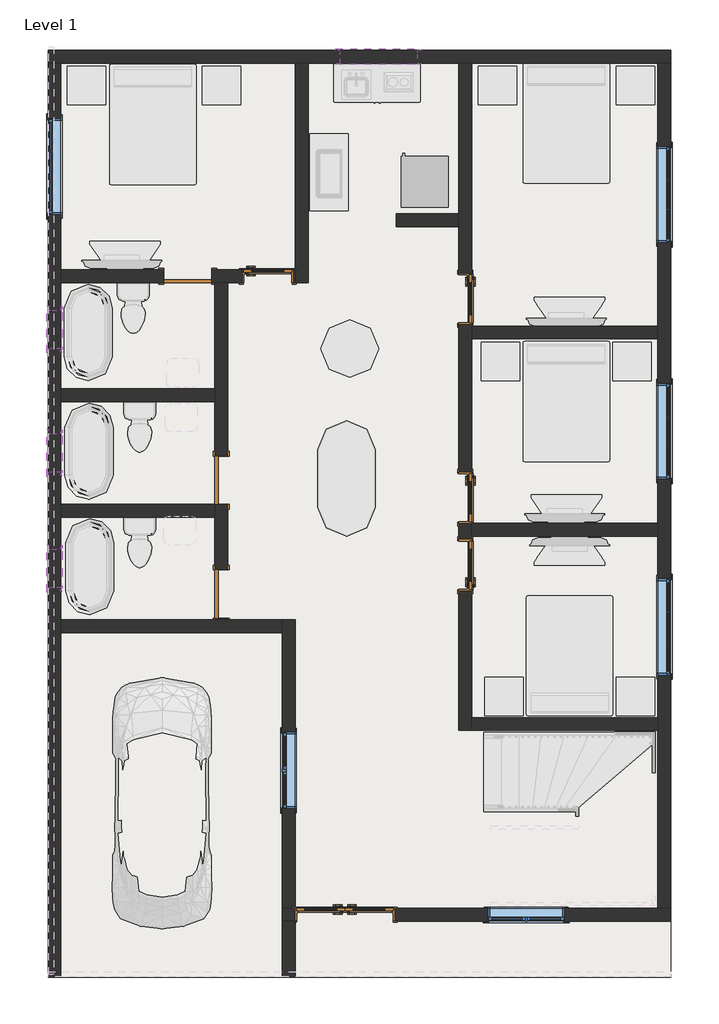
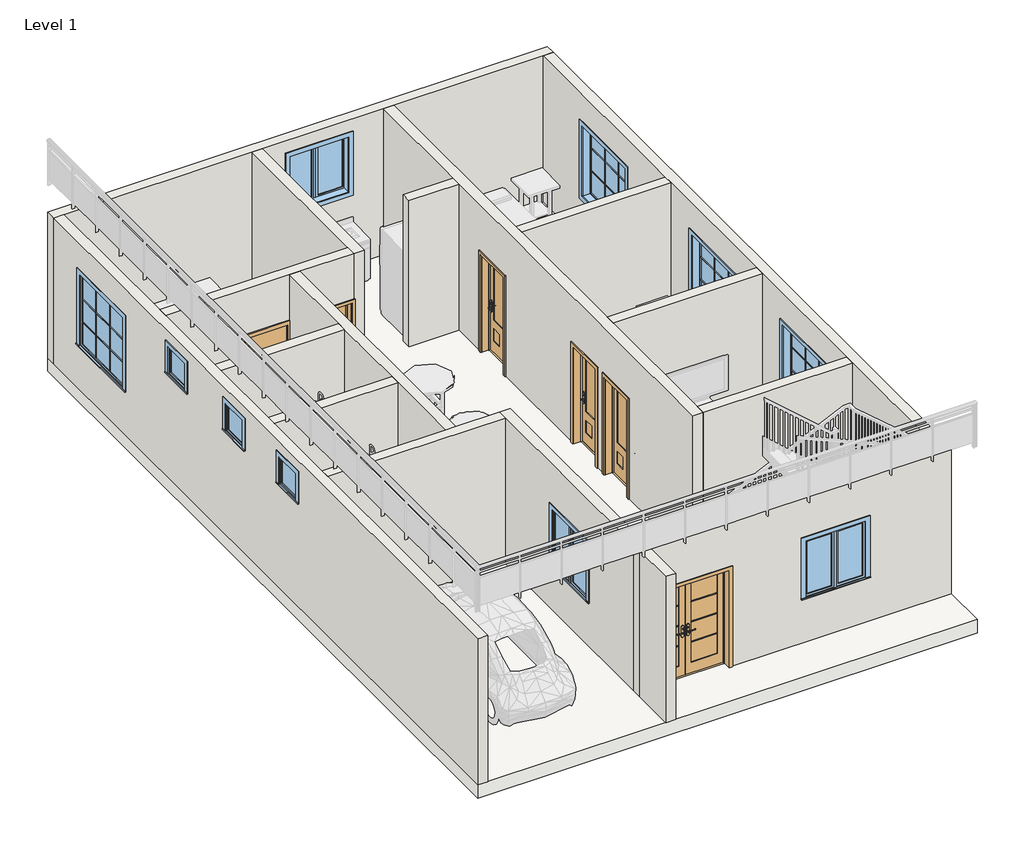
# One storey, part 1 of 4: 17 walls, 10 windows, 8 doors, 1 slab.
"""IFC4 building model written with IfcOpenShell, lengths in millimetres."""

from ifc_helpers import new_model, si_unit, frame, origin, origin_with_axes, place, context, project, spatial, polyline, outline, extrude, faceted_brep, transform, mapped, element, save
from components import door_ad59dcae, door_41326d50, door_b03bd389, door_53b1b562, window_8901c6e2, window_0862ab64, window_e41d21a6

model = new_model("IFC4")

# Units and contexts
model_context = context("Model", 3, world=origin())
ifc_project = project(units=[si_unit("LENGTHUNIT", "METRE", prefix="MILLI")], contexts=[model_context])

# Site, building, storey
site = spatial("IfcSite", under=ifc_project)
building = spatial("IfcBuilding", under=site)
storey = spatial("IfcBuildingStorey", under=building, Name="Level 1", Elevation=0.0)

# Doors
placement = place(None, origin())
door_shape = door_ad59dcae(model_context)
element("IfcDoor", 1, ObjectType="30\" x 80\"", at=placement, inside=storey, context=model_context, shape_type="MappedRepresentation", body=[
    mapped(door_shape, transform((-5611.6297602, 5281.5174997, 0.0), x_axis=(0.0, -1.0, 0.0), y_axis=(1.0, 0.0, 0.0), z_axis=(0.0, 0.0, 1.0))),
])
door_2_shape = door_41326d50(model_context)
element("IfcDoor", 2, ObjectType="30\" x 80\"", at=placement, inside=storey, context=model_context, shape_type="MappedRepresentation", body=[
    mapped(door_2_shape, transform((-5611.6297602, 6348.3174997, 0.0), x_axis=(0.0, 1.0, 0.0), y_axis=(-1.0, 0.0, 0.0), z_axis=(0.0, 0.0, 1.0))),
])
element("IfcDoor", 3, ObjectType="30\" x 80\"", at=placement, inside=storey, context=model_context, shape_type="MappedRepresentation", body=[
    mapped(door_2_shape, transform((-5611.6297602, 9497.9174997, 0.0), x_axis=(0.0, 1.0, 0.0), y_axis=(-1.0, 0.0, 0.0), z_axis=(0.0, 0.0, 1.0))),
])
element("IfcDoor", 4, ObjectType="30\" x 80\"", at=placement, inside=storey, context=model_context, shape_type="MappedRepresentation", body=[
    mapped(door_2_shape, transform((-8739.0047602, 9856.6924997, 0.0), x_axis=(-1.0, 0.0, 0.0), y_axis=(0.0, -1.0, 0.0), z_axis=(0.0, 0.0, 1.0))),
])
door_3_shape = door_b03bd389(model_context)
element("IfcDoor", 5, ObjectType="Door-Exterior-Double-Full Glass-Wood_Clad : 60\" x 80\"", at=placement, inside=storey, context=model_context, shape_type="MappedRepresentation", body=[
    mapped(door_3_shape, transform((-7519.8047602, -252.5075003, 0.0), x_axis=(1.0, 0.0, 0.0), y_axis=(0.0, 1.0, 0.0), z_axis=(0.0, 0.0, 1.0))),
])
door_4_shape = door_53b1b562(model_context)
element("IfcDoor", 6, ObjectType="Single-Flush : 30\" x 80\"", at=placement, inside=storey, context=model_context, shape_type="MappedRepresentation", body=[
    mapped(door_4_shape, transform((-9475.6047602, 4824.3174997, 0.0), x_axis=(0.0, -1.0, 0.0), y_axis=(1.0, 0.0, 0.0), z_axis=(0.0, 0.0, 1.0))),
])
element("IfcDoor", 7, ObjectType="Single-Flush : 30\" x 80\"", at=placement, inside=storey, context=model_context, shape_type="MappedRepresentation", body=[
    mapped(door_4_shape, transform((-9475.6047602, 6627.7174997, 0.0), x_axis=(0.0, -1.0, 0.0), y_axis=(1.0, 0.0, 0.0), z_axis=(0.0, 0.0, 1.0))),
])
element("IfcDoor", 8, ObjectType="Single-Flush : 30\" x 80\"", at=placement, inside=storey, context=model_context, shape_type="MappedRepresentation", body=[
    mapped(door_4_shape, transform((-10009.0047602, 9853.5174997, 0.0), x_axis=(1.0, 0.0, 0.0), y_axis=(0.0, 1.0, 0.0), z_axis=(0.0, 0.0, 1.0))),
])

# Slab
element("IfcSlab", 9, ObjectType="Wood Joist 10\" - Ceramic Tile", at=placement, inside=storey, context=model_context, shape_type="SweptSolid", body=[
    extrude(outline(polyline([(-2363.6047602, 13434.9174997), (-2363.6047602, -357.2825003), (-2363.6047602, -1246.2825003), (-12218.8047602, -1246.2825003), (-12218.8047602, 13434.9174997), (-2363.6047602, 13434.9174997)])), frame((0.0, 0.0, -273.05), z_axis=(0.0, 0.0, 1.0), x_axis=(1.0, 0.0, 0.0)), (0.0, 0.0, 1.0), 273.05),
])

# Walls
element("IfcWall", 10, ObjectType="Generic - 8\"", at=placement, inside=storey, context=model_context, shape_type="Brep", body=[
    faceted_brep([(-12015.6047602, -1246.2825003, 0.0), (-12015.6047602, 4214.7174997, 0.0), (-12015.6047602, 4417.9174997, 0.0), (-12015.6047602, 6043.5174997, 0.0), (-12015.6047602, 6246.7174997, 0.0), (-12015.6047602, 7872.3174997, 0.0), (-12015.6047602, 8075.5174997, 0.0), (-12015.6047602, 9751.9174997, 0.0), (-12015.6047602, 9955.1174997, 0.0), (-12015.6047602, 13231.7174997, 0.0), (-12015.6047602, 13231.7174997, 3048.0), (-12015.6047602, 9955.1174997, 3048.0), (-12015.6047602, 9751.9174997, 3048.0), (-12015.6047602, 8075.5174997, 3048.0), (-12015.6047602, 7872.3174997, 3048.0), (-12015.6047602, 6246.7174997, 3048.0), (-12015.6047602, 6043.5174997, 3048.0), (-12015.6047602, 4417.9174997, 3048.0), (-12015.6047602, 4214.7174997, 3048.0), (-12015.6047602, -1246.2825003, 3048.0), (-12015.6047602, 12355.4174997, 2438.4), (-12015.6047602, 12355.4174997, 914.4), (-12015.6047602, 10831.4174997, 914.4), (-12015.6047602, 10831.4174997, 2438.4), (-12015.6047602, 5535.5174997, 2768.6), (-12015.6047602, 5535.5174997, 2159.0), (-12015.6047602, 4925.9174997, 2159.0), (-12015.6047602, 4925.9174997, 2768.6), (-12015.6047602, 7364.3174997, 2768.6), (-12015.6047602, 7364.3174997, 2159.0), (-12015.6047602, 6754.7174997, 2159.0), (-12015.6047602, 6754.7174997, 2768.6), (-12015.6047602, 9320.1174997, 2768.6), (-12015.6047602, 9320.1174997, 2159.0), (-12015.6047602, 8710.5174997, 2159.0), (-12015.6047602, 8710.5174997, 2768.6), (-12218.8047602, -1246.2825003, 0.0), (-12218.8047602, -1246.2825003, 3048.0), (-12218.8047602, 13231.7174997, 3048.0), (-12218.8047602, 13231.7174997, 0.0), (-12218.8047602, 12355.4174997, 2438.4), (-12218.8047602, 10831.4174997, 2438.4), (-12218.8047602, 10831.4174997, 914.4), (-12218.8047602, 12355.4174997, 914.4), (-12218.8047602, 5535.5174997, 2768.6), (-12218.8047602, 4925.9174997, 2768.6), (-12218.8047602, 4925.9174997, 2159.0), (-12218.8047602, 5535.5174997, 2159.0), (-12218.8047602, 7364.3174997, 2768.6), (-12218.8047602, 6754.7174997, 2768.6), (-12218.8047602, 6754.7174997, 2159.0), (-12218.8047602, 7364.3174997, 2159.0), (-12218.8047602, 9320.1174997, 2768.6), (-12218.8047602, 8710.5174997, 2768.6), (-12218.8047602, 8710.5174997, 2159.0), (-12218.8047602, 9320.1174997, 2159.0)], [[[0, 1, 2, 3, 4, 5, 6, 7, 8, 9, 10, 11, 12, 13, 14, 15, 16, 17, 18, 19], [20, 21, 22, 23], [24, 25, 26, 27], [28, 29, 30, 31], [32, 33, 34, 35]], [[36, 37, 38, 39], [40, 41, 42, 43], [44, 45, 46, 47], [48, 49, 50, 51], [52, 53, 54, 55]], [[9, 8, 7, 6, 5, 4, 3, 2, 1, 0, 36, 39]], [[0, 19, 37, 36]], [[10, 9, 39, 38]], [[19, 18, 17, 16, 15, 14, 13, 12, 11, 10, 38, 37]], [[21, 20, 40, 43]], [[22, 21, 43, 42]], [[23, 22, 42, 41]], [[20, 23, 41, 40]], [[25, 24, 44, 47]], [[26, 25, 47, 46]], [[27, 26, 46, 45]], [[24, 27, 45, 44]], [[29, 28, 48, 51]], [[30, 29, 51, 50]], [[31, 30, 50, 49]], [[28, 31, 49, 48]], [[33, 32, 52, 55]], [[34, 33, 55, 54]], [[35, 34, 54, 53]], [[32, 35, 53, 52]]]),
])
element("IfcWall", 11, ObjectType="Generic - 8\"", at=placement, inside=storey, context=model_context, shape_type="Brep", body=[
    faceted_brep([(-2566.8047602, 13231.7174997, 0.0), (-2566.8047602, 9066.1174997, 0.0), (-2566.8047602, 8862.9174997, 0.0), (-2566.8047602, 5941.9174997, 0.0), (-2566.8047602, 5738.7174997, 0.0), (-2566.8047602, 2868.5174997, 0.0), (-2566.8047602, 2665.3174997, 0.0), (-2566.8047602, -154.0825003, 0.0), (-2566.8047602, -154.0825003, 3048.0), (-2566.8047602, 2665.3174997, 3048.0), (-2566.8047602, 2868.5174997, 3048.0), (-2566.8047602, 5738.7174997, 3048.0), (-2566.8047602, 5941.9174997, 3048.0), (-2566.8047602, 8862.9174997, 3048.0), (-2566.8047602, 9066.1174997, 3048.0), (-2566.8047602, 13231.7174997, 3048.0), (-2566.8047602, 3541.6174997, 2438.4), (-2566.8047602, 3541.6174997, 914.4), (-2566.8047602, 5065.6174997, 914.4), (-2566.8047602, 5065.6174997, 2438.4), (-2566.8047602, 6640.4174997, 2438.4), (-2566.8047602, 6640.4174997, 914.4), (-2566.8047602, 8164.4174997, 914.4), (-2566.8047602, 8164.4174997, 2438.4), (-2566.8047602, 10386.9174997, 2438.4), (-2566.8047602, 10386.9174997, 914.4), (-2566.8047602, 11910.9174997, 914.4), (-2566.8047602, 11910.9174997, 2438.4), (-2363.6047602, 13231.7174997, 0.0), (-2363.6047602, 13231.7174997, 3048.0), (-2363.6047602, -154.0825003, 3048.0), (-2363.6047602, -154.0825003, 0.0), (-2363.6047602, 3541.6174997, 2438.4), (-2363.6047602, 5065.6174997, 2438.4), (-2363.6047602, 5065.6174997, 914.4), (-2363.6047602, 3541.6174997, 914.4), (-2363.6047602, 6640.4174997, 2438.4), (-2363.6047602, 8164.4174997, 2438.4), (-2363.6047602, 8164.4174997, 914.4), (-2363.6047602, 6640.4174997, 914.4), (-2363.6047602, 10386.9174997, 2438.4), (-2363.6047602, 11910.9174997, 2438.4), (-2363.6047602, 11910.9174997, 914.4), (-2363.6047602, 10386.9174997, 914.4)], [[[0, 1, 2, 3, 4, 5, 6, 7, 8, 9, 10, 11, 12, 13, 14, 15], [16, 17, 18, 19], [20, 21, 22, 23], [24, 25, 26, 27]], [[28, 29, 30, 31], [32, 33, 34, 35], [36, 37, 38, 39], [40, 41, 42, 43]], [[7, 6, 5, 4, 3, 2, 1, 0, 28, 31]], [[8, 7, 31, 30]], [[0, 15, 29, 28]], [[15, 14, 13, 12, 11, 10, 9, 8, 30, 29]], [[17, 16, 32, 35]], [[18, 17, 35, 34]], [[19, 18, 34, 33]], [[16, 19, 33, 32]], [[21, 20, 36, 39]], [[22, 21, 39, 38]], [[23, 22, 38, 37]], [[20, 23, 37, 36]], [[25, 24, 40, 43]], [[26, 25, 43, 42]], [[27, 26, 42, 41]], [[24, 27, 41, 40]]]),
])
element("IfcWall", 12, ObjectType="Generic - 8\"", at=placement, inside=storey, context=model_context, shape_type="Brep", body=[
    faceted_brep([(-2363.6047602, -154.0825003, 3048.0), (-2363.6047602, -154.0825003, 0.0), (-2566.8047602, -154.0825003, 0.0), (-6732.4047602, -154.0825003, 0.0), (-6732.4047602, -154.0825003, 2057.4), (-8307.2047602, -154.0825003, 2057.4), (-8307.2047602, -154.0825003, 0.0), (-8510.4047602, -154.0825003, 0.0), (-8510.4047602, -154.0825003, 3048.0), (-8307.2047602, -154.0825003, 3048.0), (-2566.8047602, -154.0825003, 3048.0), (-5259.2047602, -154.0825003, 2133.6), (-5259.2047602, -154.0825003, 914.4), (-4040.0047602, -154.0825003, 914.4), (-4040.0047602, -154.0825003, 2133.6), (-2363.6047602, -357.2825003, 0.0), (-2363.6047602, -357.2825003, 3048.0), (-8307.2047602, -357.2825003, 3048.0), (-8510.4047602, -357.2825003, 3048.0), (-8510.4047602, -357.2825003, 0.0), (-8307.2047602, -357.2825003, 0.0), (-8307.2047602, -357.2825003, 2057.4), (-6732.4047602, -357.2825003, 2057.4), (-6732.4047602, -357.2825003, 0.0), (-5259.2047602, -357.2825003, 2133.6), (-4040.0047602, -357.2825003, 2133.6), (-4040.0047602, -357.2825003, 914.4), (-5259.2047602, -357.2825003, 914.4)], [[[0, 1, 2, 3, 4, 5, 6, 7, 8, 9, 10], [11, 12, 13, 14]], [[15, 16, 17, 18, 19, 20, 21, 22, 23], [24, 25, 26, 27]], [[1, 15, 23, 3, 2]], [[19, 7, 6, 20]], [[1, 0, 16, 15]], [[8, 7, 19, 18]], [[0, 10, 9, 8, 18, 17, 16]], [[22, 4, 3, 23]], [[4, 22, 21, 5]], [[5, 21, 20, 6]], [[12, 11, 24, 27]], [[13, 12, 27, 26]], [[14, 13, 26, 25]], [[11, 14, 25, 24]]]),
])
element("IfcWall", 13, ObjectType="Generic - 8\"", at=placement, inside=storey, context=model_context, shape_type="Brep", body=[
    faceted_brep([(-12218.8047602, 13231.7174997, 0.0), (-12015.6047602, 13231.7174997, 0.0), (-8307.2047602, 13231.7174997, 0.0), (-8104.0047602, 13231.7174997, 0.0), (-5716.4047602, 13231.7174997, 0.0), (-5513.2047602, 13231.7174997, 0.0), (-2566.8047602, 13231.7174997, 0.0), (-2363.6047602, 13231.7174997, 0.0), (-2363.6047602, 13231.7174997, 3048.0), (-2566.8047602, 13231.7174997, 3048.0), (-5513.2047602, 13231.7174997, 3048.0), (-5716.4047602, 13231.7174997, 3048.0), (-8104.0047602, 13231.7174997, 3048.0), (-8307.2047602, 13231.7174997, 3048.0), (-12015.6047602, 13231.7174997, 3048.0), (-12218.8047602, 13231.7174997, 3048.0), (-6376.8047602, 13231.7174997, 2743.2), (-6376.8047602, 13231.7174997, 1524.0), (-7596.0047602, 13231.7174997, 1524.0), (-7596.0047602, 13231.7174997, 2743.2), (-12218.8047602, 13434.9174997, 0.0), (-12218.8047602, 13434.9174997, 3048.0), (-2363.6047602, 13434.9174997, 3048.0), (-2363.6047602, 13434.9174997, 0.0), (-6376.8047602, 13434.9174997, 2743.2), (-7596.0047602, 13434.9174997, 2743.2), (-7596.0047602, 13434.9174997, 1524.0), (-6376.8047602, 13434.9174997, 1524.0)], [[[0, 1, 2, 3, 4, 5, 6, 7, 8, 9, 10, 11, 12, 13, 14, 15], [16, 17, 18, 19]], [[20, 21, 22, 23], [24, 25, 26, 27]], [[7, 6, 5, 4, 3, 2, 1, 0, 20, 23]], [[0, 15, 21, 20]], [[8, 7, 23, 22]], [[15, 14, 13, 12, 11, 10, 9, 8, 22, 21]], [[17, 16, 24, 27]], [[18, 17, 27, 26]], [[19, 18, 26, 25]], [[16, 19, 25, 24]]]),
])
element("IfcWall", 14, ObjectType="Generic - 8\"", at=placement, inside=storey, context=model_context, shape_type="Brep", body=[
    faceted_brep([(-8307.2047602, -154.0825003, 0.0), (-8307.2047602, 4417.9174997, 0.0), (-8307.2047602, 4417.9174997, 3048.0), (-8307.2047602, -154.0825003, 3048.0), (-8307.2047602, -154.0825003, 2057.4), (-8307.2047602, 2639.9174997, 2133.6), (-8307.2047602, 2639.9174997, 914.4), (-8307.2047602, 1420.7174997, 914.4), (-8307.2047602, 1420.7174997, 2133.6), (-8510.4047602, -154.0825003, 0.0), (-8510.4047602, -154.0825003, 3048.0), (-8510.4047602, 4214.7174997, 3048.0), (-8510.4047602, 4417.9174997, 3048.0), (-8510.4047602, 4417.9174997, 0.0), (-8510.4047602, 4214.7174997, 0.0), (-8510.4047602, 2639.9174997, 2133.6), (-8510.4047602, 1420.7174997, 2133.6), (-8510.4047602, 1420.7174997, 914.4), (-8510.4047602, 2639.9174997, 914.4)], [[[0, 1, 2, 3, 4], [5, 6, 7, 8]], [[9, 10, 11, 12, 13, 14], [15, 16, 17, 18]], [[1, 0, 9, 14, 13]], [[0, 4, 3, 10, 9]], [[2, 1, 13, 12]], [[3, 2, 12, 11, 10]], [[6, 5, 15, 18]], [[7, 6, 18, 17]], [[8, 7, 17, 16]], [[5, 8, 16, 15]]]),
])
element("IfcWall", 15, ObjectType="Generic - 8\"", at=placement, inside=storey, context=model_context, shape_type="Brep", body=[
    faceted_brep([(-8510.4047602, 4417.9174997, 0.0), (-9374.0047602, 4417.9174997, 0.0), (-9577.2047602, 4417.9174997, 0.0), (-12015.6047602, 4417.9174997, 0.0), (-12015.6047602, 4417.9174997, 3048.0), (-9577.2047602, 4417.9174997, 3048.0), (-9374.0047602, 4417.9174997, 3048.0), (-8510.4047602, 4417.9174997, 3048.0), (-8510.4047602, 4214.7174997, 0.0), (-8510.4047602, 4214.7174997, 3048.0), (-12015.6047602, 4214.7174997, 3048.0), (-12015.6047602, 4214.7174997, 0.0)], [[[0, 1, 2, 3, 4, 5, 6, 7]], [[8, 9, 10, 11]], [[3, 2, 1, 0, 8, 11]], [[0, 7, 9, 8]], [[4, 3, 11, 10]], [[7, 6, 5, 4, 10, 9]]]),
])
element("IfcWall", 16, ObjectType="Generic - 8\"", at=placement, inside=storey, context=model_context, shape_type="Brep", body=[
    faceted_brep([(-8307.2047602, 13231.7174997, 0.0), (-8307.2047602, 9955.1174997, 0.0), (-8307.2047602, 9751.9174997, 0.0), (-8307.2047602, 9751.9174997, 3048.0), (-8307.2047602, 9955.1174997, 3048.0), (-8307.2047602, 13231.7174997, 3048.0), (-8104.0047602, 13231.7174997, 0.0), (-8104.0047602, 13231.7174997, 3048.0), (-8104.0047602, 9751.9174997, 3048.0), (-8104.0047602, 9751.9174997, 0.0)], [[[0, 1, 2, 3, 4, 5]], [[6, 7, 8, 9]], [[2, 1, 0, 6, 9]], [[0, 5, 7, 6]], [[3, 2, 9, 8]], [[5, 4, 3, 8, 7]]]),
])
element("IfcWall", 17, ObjectType="Generic - 8\"", at=placement, inside=storey, context=model_context, shape_type="Brep", body=[
    faceted_brep([(-8307.2047602, 9955.1174997, 3048.0), (-8307.2047602, 9955.1174997, 0.0), (-8332.6047602, 9955.1174997, 0.0), (-8332.6047602, 9955.1174997, 2057.4), (-9145.4047602, 9955.1174997, 2057.4), (-9145.4047602, 9955.1174997, 0.0), (-9628.0047602, 9955.1174997, 0.0), (-9628.0047602, 9955.1174997, 2032.0), (-10390.0047602, 9955.1174997, 2032.0), (-10390.0047602, 9955.1174997, 0.0), (-12015.6047602, 9955.1174997, 0.0), (-12015.6047602, 9955.1174997, 3048.0), (-8307.2047602, 9751.9174997, 0.0), (-8307.2047602, 9751.9174997, 3048.0), (-9374.0047602, 9751.9174997, 3048.0), (-9577.2047602, 9751.9174997, 3048.0), (-12015.6047602, 9751.9174997, 3048.0), (-12015.6047602, 9751.9174997, 0.0), (-10390.0047602, 9751.9174997, 0.0), (-10390.0047602, 9751.9174997, 2032.0), (-9628.0047602, 9751.9174997, 2032.0), (-9628.0047602, 9751.9174997, 0.0), (-9577.2047602, 9751.9174997, 0.0), (-9374.0047602, 9751.9174997, 0.0), (-9145.4047602, 9751.9174997, 0.0), (-9145.4047602, 9751.9174997, 2057.4), (-8332.6047602, 9751.9174997, 2057.4), (-8332.6047602, 9751.9174997, 0.0)], [[[0, 1, 2, 3, 4, 5, 6, 7, 8, 9, 10, 11]], [[12, 13, 14, 15, 16, 17, 18, 19, 20, 21, 22, 23, 24, 25, 26, 27]], [[1, 12, 27, 2]], [[17, 10, 9, 18]], [[21, 6, 5, 24, 23, 22]], [[1, 0, 13, 12]], [[11, 10, 17, 16]], [[7, 6, 21, 20]], [[8, 7, 20, 19]], [[9, 8, 19, 18]], [[0, 11, 16, 15, 14, 13]], [[4, 25, 24, 5]], [[25, 4, 3, 26]], [[26, 3, 2, 27]]]),
])
element("IfcWall", 18, ObjectType="Generic - 8\"", at=placement, inside=storey, context=model_context, shape_type="Brep", body=[
    faceted_brep([(-9577.2047602, 6246.7174997, 2032.0), (-9577.2047602, 6246.7174997, 0.0), (-9577.2047602, 6043.5174997, 0.0), (-9577.2047602, 5205.3174997, 0.0), (-9577.2047602, 5205.3174997, 2032.0), (-9577.2047602, 4443.3174997, 2032.0), (-9577.2047602, 4443.3174997, 0.0), (-9577.2047602, 4417.9174997, 0.0), (-9577.2047602, 4417.9174997, 3048.0), (-9577.2047602, 6043.5174997, 3048.0), (-9577.2047602, 6246.7174997, 3048.0), (-9577.2047602, 7872.3174997, 3048.0), (-9577.2047602, 8075.5174997, 3048.0), (-9577.2047602, 9751.9174997, 3048.0), (-9577.2047602, 9751.9174997, 0.0), (-9577.2047602, 8075.5174997, 0.0), (-9577.2047602, 7872.3174997, 0.0), (-9577.2047602, 7008.7174997, 0.0), (-9577.2047602, 7008.7174997, 2032.0), (-9374.0047602, 5205.3174997, 0.0), (-9374.0047602, 6246.7174997, 0.0), (-9374.0047602, 6246.7174997, 2032.0), (-9374.0047602, 7008.7174997, 2032.0), (-9374.0047602, 7008.7174997, 0.0), (-9374.0047602, 9751.9174997, 0.0), (-9374.0047602, 9751.9174997, 3048.0), (-9374.0047602, 4417.9174997, 3048.0), (-9374.0047602, 4417.9174997, 0.0), (-9374.0047602, 4443.3174997, 0.0), (-9374.0047602, 4443.3174997, 2032.0), (-9374.0047602, 5205.3174997, 2032.0)], [[[0, 1, 2, 3, 4, 5, 6, 7, 8, 9, 10, 11, 12, 13, 14, 15, 16, 17, 18]], [[19, 20, 21, 22, 23, 24, 25, 26, 27, 28, 29, 30]], [[7, 6, 28, 27]], [[3, 2, 1, 20, 19]], [[17, 16, 15, 14, 24, 23]], [[8, 7, 27, 26]], [[14, 13, 25, 24]], [[29, 28, 6, 5]], [[30, 29, 5, 4]], [[19, 30, 4, 3]], [[21, 20, 1, 0]], [[22, 21, 0, 18]], [[23, 22, 18, 17]], [[13, 12, 11, 10, 9, 8, 26, 25]]]),
])
element("IfcWall", 19, ObjectType="Generic - 8\"", at=placement, inside=storey, context=model_context, shape_type="Brep", body=[
    faceted_brep([(-12015.6047602, 6043.5174997, 0.0), (-9577.2047602, 6043.5174997, 0.0), (-9577.2047602, 6043.5174997, 3048.0), (-12015.6047602, 6043.5174997, 3048.0), (-12015.6047602, 6246.7174997, 0.0), (-12015.6047602, 6246.7174997, 3048.0), (-9577.2047602, 6246.7174997, 3048.0), (-9577.2047602, 6246.7174997, 2032.0), (-9577.2047602, 6246.7174997, 0.0)], [[[0, 1, 2, 3]], [[4, 5, 6, 7, 8]], [[1, 0, 4, 8]], [[0, 3, 5, 4]], [[2, 1, 8, 7, 6]], [[3, 2, 6, 5]]]),
])
element("IfcWall", 20, ObjectType="Generic - 8\"", at=placement, inside=storey, context=model_context, shape_type="SweptSolid", body=[
    extrude(outline(polyline([(-9577.2047602, 7872.3174997), (-12015.6047602, 7872.3174997), (-12015.6047602, 8075.5174997), (-9577.2047602, 8075.5174997), (-9577.2047602, 7872.3174997)])), origin_with_axes(), (0.0, 0.0, 1.0), 3048.0),
])
element("IfcWall", 21, ObjectType="Generic - 8\"", at=placement, inside=storey, context=model_context, shape_type="Brep", body=[
    faceted_brep([(-5716.4047602, 13231.7174997, 3048.0), (-5716.4047602, 13231.7174997, 0.0), (-5716.4047602, 10844.1174997, 0.0), (-5716.4047602, 10640.9174997, 0.0), (-5716.4047602, 9904.3174997, 0.0), (-5716.4047602, 9904.3174997, 2057.4), (-5716.4047602, 9091.5174997, 2057.4), (-5716.4047602, 9091.5174997, 0.0), (-5716.4047602, 6754.7174997, 0.0), (-5716.4047602, 6754.7174997, 2057.4), (-5716.4047602, 5941.9174997, 2057.4), (-5716.4047602, 5941.9174997, 0.0), (-5716.4047602, 5687.9174997, 0.0), (-5716.4047602, 5687.9174997, 2057.4), (-5716.4047602, 4875.1174997, 2057.4), (-5716.4047602, 4875.1174997, 0.0), (-5716.4047602, 2665.3174997, 0.0), (-5716.4047602, 2665.3174997, 3048.0), (-5716.4047602, 10640.9174997, 3048.0), (-5716.4047602, 10844.1174997, 3048.0), (-5513.2047602, 13231.7174997, 0.0), (-5513.2047602, 13231.7174997, 3048.0), (-5513.2047602, 9066.1174997, 3048.0), (-5513.2047602, 8862.9174997, 3048.0), (-5513.2047602, 5941.9174997, 3048.0), (-5513.2047602, 5738.7174997, 3048.0), (-5513.2047602, 2868.5174997, 3048.0), (-5513.2047602, 2665.3174997, 3048.0), (-5513.2047602, 2665.3174997, 0.0), (-5513.2047602, 2868.5174997, 0.0), (-5513.2047602, 4875.1174997, 0.0), (-5513.2047602, 4875.1174997, 2057.4), (-5513.2047602, 5687.9174997, 2057.4), (-5513.2047602, 5687.9174997, 0.0), (-5513.2047602, 5738.7174997, 0.0), (-5513.2047602, 5941.9174997, 0.0), (-5513.2047602, 5941.9174997, 2057.4), (-5513.2047602, 6754.7174997, 2057.4), (-5513.2047602, 6754.7174997, 0.0), (-5513.2047602, 8862.9174997, 0.0), (-5513.2047602, 9066.1174997, 0.0), (-5513.2047602, 9091.5174997, 0.0), (-5513.2047602, 9091.5174997, 2057.4), (-5513.2047602, 9904.3174997, 2057.4), (-5513.2047602, 9904.3174997, 0.0)], [[[0, 1, 2, 3, 4, 5, 6, 7, 8, 9, 10, 11, 12, 13, 14, 15, 16, 17, 18, 19]], [[20, 21, 22, 23, 24, 25, 26, 27, 28, 29, 30, 31, 32, 33, 34, 35, 36, 37, 38, 39, 40, 41, 42, 43, 44]], [[1, 20, 44, 4, 3, 2]], [[28, 16, 15, 30, 29]], [[33, 12, 11, 35, 34]], [[38, 8, 7, 41, 40, 39]], [[1, 0, 21, 20]], [[17, 16, 28, 27]], [[0, 19, 18, 17, 27, 26, 25, 24, 23, 22, 21]], [[14, 31, 30, 15]], [[31, 14, 13, 32]], [[32, 13, 12, 33]], [[37, 9, 8, 38]], [[9, 37, 36, 10]], [[10, 36, 35, 11]], [[43, 5, 4, 44]], [[5, 43, 42, 6]], [[6, 42, 41, 7]]]),
])
element("IfcWall", 22, ObjectType="Generic - 8\"", at=placement, inside=storey, context=model_context, shape_type="SweptSolid", body=[
    extrude(outline(polyline([(-6707.0047602, 10844.1174997), (-5716.4047602, 10844.1174997), (-5716.4047602, 10640.9174997), (-6707.0047602, 10640.9174997), (-6707.0047602, 10844.1174997)])), origin_with_axes(), (0.0, 0.0, 1.0), 3048.0),
])
element("IfcWall", 23, ObjectType="Generic - 8\"", at=placement, inside=storey, context=model_context, shape_type="SweptSolid", body=[
    extrude(outline(polyline([(-2566.8047602, 8862.9174997), (-5513.2047602, 8862.9174997), (-5513.2047602, 9066.1174997), (-2566.8047602, 9066.1174997), (-2566.8047602, 8862.9174997)])), origin_with_axes(), (0.0, 0.0, 1.0), 3048.0),
])
element("IfcWall", 24, ObjectType="Generic - 8\"", at=placement, inside=storey, context=model_context, shape_type="SweptSolid", body=[
    extrude(outline(polyline([(-2566.8047602, 5738.7174997), (-5513.2047602, 5738.7174997), (-5513.2047602, 5941.9174997), (-2566.8047602, 5941.9174997), (-2566.8047602, 5738.7174997)])), origin_with_axes(), (0.0, 0.0, 1.0), 3048.0),
])
element("IfcWall", 25, ObjectType="Generic - 8\"", at=placement, inside=storey, context=model_context, shape_type="SweptSolid", body=[
    extrude(outline(polyline([(-2566.8047602, 2665.3174997), (-5513.2047602, 2665.3174997), (-5513.2047602, 2868.5174997), (-2566.8047602, 2868.5174997), (-2566.8047602, 2665.3174997)])), origin_with_axes(), (0.0, 0.0, 1.0), 3048.0),
])
element("IfcWall", 26, ObjectType="Generic - 8\"", at=placement, inside=storey, context=model_context, shape_type="Brep", body=[
    faceted_brep([(-8307.2047602, -1246.2825003, 0.0), (-8307.2047602, -357.2825003, 0.0), (-8307.2047602, -357.2825003, 2057.4), (-8307.2047602, -357.2825003, 3048.0), (-8307.2047602, -1246.2825003, 3048.0), (-8510.4047602, -1246.2825003, 0.0), (-8510.4047602, -1246.2825003, 3048.0), (-8510.4047602, -357.2825003, 3048.0), (-8510.4047602, -357.2825003, 0.0)], [[[0, 1, 2, 3, 4]], [[5, 6, 7, 8]], [[1, 0, 5, 8]], [[0, 4, 6, 5]], [[3, 2, 1, 8, 7]], [[4, 3, 7, 6]]]),
])

# Windows
window_shape = window_8901c6e2(model_context)
element("IfcWindow", 27, ObjectType="Casement 3x3 with Trim : 60\" x 60\"", at=placement, inside=storey, context=model_context, shape_type="MappedRepresentation", body=[
    mapped(window_shape, transform((-2465.2047602, 4303.6174997, 609.6), x_axis=(0.0, -1.0, 0.0), y_axis=(1.0, 0.0, 0.0), z_axis=(0.0, 0.0, 1.0))),
])
element("IfcWindow", 28, ObjectType="Casement 3x3 with Trim : 60\" x 60\"", at=placement, inside=storey, context=model_context, shape_type="MappedRepresentation", body=[
    mapped(window_shape, transform((-2465.2047602, 7402.4174997, 609.6), x_axis=(0.0, -1.0, 0.0), y_axis=(1.0, 0.0, 0.0), z_axis=(0.0, 0.0, 1.0))),
])
element("IfcWindow", 29, ObjectType="Casement 3x3 with Trim : 60\" x 60\"", at=placement, inside=storey, context=model_context, shape_type="MappedRepresentation", body=[
    mapped(window_shape, transform((-2465.2047602, 11148.9174997, 609.6), x_axis=(0.0, -1.0, 0.0), y_axis=(1.0, 0.0, 0.0), z_axis=(0.0, 0.0, 1.0))),
])
element("IfcWindow", 30, ObjectType="Casement 3x3 with Trim : 60\" x 60\"", at=placement, inside=storey, context=model_context, shape_type="MappedRepresentation", body=[
    mapped(window_shape, transform((-12117.2047602, 11593.4174997, 609.6), x_axis=(0.0, 1.0, 0.0), y_axis=(-1.0, 0.0, 0.0), z_axis=(0.0, 0.0, 1.0))),
])
window_2_shape = window_0862ab64(model_context)
element("IfcWindow", 31, ObjectType="Casement Dbl with Trim : 48\" x 48\"", at=placement, inside=storey, context=model_context, shape_type="MappedRepresentation", body=[
    mapped(window_2_shape, transform((-6986.4047602, 13314.2674997, 609.6), x_axis=(1.0, 0.0, 0.0), y_axis=(0.0, 1.0, 0.0), z_axis=(0.0, 0.0, 1.0))),
])
element("IfcWindow", 32, ObjectType="Casement Dbl with Trim : 48\" x 48\"", at=placement, inside=storey, context=model_context, shape_type="MappedRepresentation", body=[
    mapped(window_2_shape, transform((-4649.6047602, -236.6325003, 0.0), x_axis=(-1.0, 0.0, 0.0), y_axis=(0.0, -1.0, 0.0), z_axis=(0.0, 0.0, 1.0))),
])
element("IfcWindow", 33, ObjectType="Casement Dbl with Trim : 48\" x 48\"", at=placement, inside=storey, context=model_context, shape_type="MappedRepresentation", body=[
    mapped(window_2_shape, transform((-8389.7547602, 2030.3174997, 0.0), x_axis=(0.0, 1.0, 0.0), y_axis=(-1.0, 0.0, 0.0), z_axis=(0.0, 0.0, 1.0))),
])
window_3_shape = window_e41d21a6(model_context)
element("IfcWindow", 34, ObjectType="Transom with Trim : 24\" x 24\"", at=placement, inside=storey, context=model_context, shape_type="MappedRepresentation", body=[
    mapped(window_3_shape, transform((-12117.2047602, 5268.8174997, 0.0), x_axis=(0.0, 1.0, 0.0), y_axis=(-1.0, 0.0, 0.0), z_axis=(0.0, 0.0, 1.0))),
])
element("IfcWindow", 35, ObjectType="Transom with Trim : 24\" x 24\"", at=placement, inside=storey, context=model_context, shape_type="MappedRepresentation", body=[
    mapped(window_3_shape, transform((-12117.2047602, 7097.6174997, 0.0), x_axis=(0.0, 1.0, 0.0), y_axis=(-1.0, 0.0, 0.0), z_axis=(0.0, 0.0, 1.0))),
])
element("IfcWindow", 36, ObjectType="Transom with Trim : 24\" x 24\"", at=placement, inside=storey, context=model_context, shape_type="MappedRepresentation", body=[
    mapped(window_3_shape, transform((-12117.2047602, 9053.4174997, 0.0), x_axis=(0.0, 1.0, 0.0), y_axis=(-1.0, 0.0, 0.0), z_axis=(0.0, 0.0, 1.0))),
])

save(model, "model.ifc")

# Revit data of these elements
# Type "30\" x 80\""
#   Type Mark = "9"
#   Assembly Code = "B2030100"
#   Analytic Construction = "French door, wood frame with single glass"
#   Threshold Offset [instance default] = 0' - 0 1/2"
#   Thickness = 0' - 1 3/8"
#   Thermal Resistance (R) = 1.0696 (h·ft²·°F)/BTU
#   Swing Angle [instance default] = 90.00°
#   Stiles = 0' - 4 3/4"
#   Rough Width = 2' - 8"
#   Rough Height = 6' - 9"
#   Radius = 1' - 1.00625"
#   Lock Rail = 0' - 7 1/8"
#   Height = 6' - 8"
#   Width = 2' - 6"
#   Heat Transfer Coefficient (U) = 0.9350 BTU/(h·ft²·°F)
#   Door Offset [instance default] = 0' - 0"
#   Bottom Rail = 0' - 9 1/2"
#   Threshold [instance default] = yes
#   Function = 1
#   Exterior Trim [instance default] = yes
#   Trim Material = Cherry
#   Threshold Material = Cherry
#   Panel Material = Cherry
#   Glazing = Glass
#   Frame Material = Cherry
#   Door Handle Material = Aluminum
#   Visual Light Transmittance = 0
#   Solar Heat Gain Coefficient = 0
#   Wall Closure = (empty or 0)
#   Construction Type = (empty or 0)
# Type "Door-Exterior-Double-Full Glass-Wood_Clad : 60\" x 80\""
#   Type Mark = "8"
#   Assembly Code = "B2030100"
#   Analytic Construction = "French door, wood frame with double glass"
#   Top Rail = 0' - 4 11/16"
#   Threshold Offset [instance default] = 0' - 0 1/2"
#   Thickness = 0' - 1 3/8"
#   Thermal Resistance (R) = 1.9158 (h·ft²·°F)/BTU
#   Swing Angle [instance default] = 90.00°
#   Stiles = 0' - 4 3/4"
#   Rough Width = 5' - 2"
#   Rough Height = 6' - 9"
#   Panel Width = 2' - 6"
#   Door Offset [instance default] = 0' - 0"
#   Height = 6' - 8"
#   Width = 5' - 0"
#   Heat Transfer Coefficient (U) = 0.5220 BTU/(h·ft²·°F)
#   Bottom Rail = 0' - 9 1/8"
#   Exterior Trim [instance default] = yes
#   Threshold [instance default] = yes
#   Show Grill [instance default] = yes
#   Function = 1
#   Trim Material = Cherry
#   Threshold Material = Cherry
#   Panel Material = Cherry
#   Glazing = Glass
#   Frame Material = Cherry
#   Door Handle Material = Aluminum
#   Visual Light Transmittance = 0
#   Solar Heat Gain Coefficient = 0
#   Wall Closure = (empty or 0)
#   Construction Type = (empty or 0)
# Type "Single-Flush : 30\" x 80\""
#   Type Mark = "5"
#   Construction Type Id = "MDOOR"
#   Assembly Code = "C1020"
#   Analytic Construction = "Metal"
#   Thickness = 0' - 2"
#   Heat Transfer Coefficient (U) = 0.651978 BTU/(h·ft²·°F)
#   Height = 6' - 8"
#   Trim Projection Ext = 0' - 1"
#   Trim Projection Int = 0' - 1"
#   Trim Width = 0' - 3"
#   Width = 2' - 6"
#   Define Thermal Properties by = 1
#   Door Material = Door - Panel
#   Frame Material = Door - Frame
#   Visual Light Transmittance = 0
#   Solar Heat Gain Coefficient = 0
#   Function = (empty or 0)
#   Wall Closure = (empty or 0)
# Type "Wood Joist 10\" - Ceramic Tile"
#   Assembly Code = "B1010"
#   Function = 0
#   Layers, outside or top first: 0' - 0 1/4" "Tile, Mosaic, Gray" (function 5); 0' - 0 1/2" "Concrete, Cast-in-Place gray" (function 4); 0' - 0 3/4" "Plywood, Sheathing" (function 1); 0' - 9 1/4" "Structure, Wood Joist/Rafter Layer" (function 1)
# Type "Generic - 8\""
#   Assembly Code = "B2010"
#   Layers, outside or top first: 0' - 8" "Brick, Common" (function 1)
# Type "Casement 3x3 with Trim : 60\" x 60\""
#   Type Mark = "12"
#   Construction Type Id = "GSP4R"
#   Assembly Code = "B2020100"
#   Analytic Construction = "1/8 in Pilkington single glazing"
#   Visual Light Transmittance = 0.9
#   Solar Heat Gain Coefficient = 0.78
#   Heat Transfer Coefficient (U) = 0.6496 BTU/(h·ft²·°F)
#   Height = 5' - 0"
#   Default Sill Height = 1' - 0"
#   Trim Projection - Ext. = 0' - 0 1/2"
#   Trim Projection - Int. = 0' - 0 3/4"
#   Trim Width - Exterior = 0' - 3 1/2"
#   Trim Width - Interior = 0' - 3 1/2"
#   Width = 5' - 0"
#   Window Inset = 0' - 0 3/4"
#   Define Thermal Properties by = 1
#   Glass Pane Material = Glass
#   Sash Material = Sash
#   Trim Exterior Material = Trim
#   Trim Interior Material = Trim
#   Wall Closure = (empty or 0)
# Type "Casement Dbl with Trim : 48\" x 48\""
#   Type Mark = "23"
#   Construction Type Id = "GSP4R"
#   Assembly Code = "B2020100"
#   Analytic Construction = "1/8 in Pilkington single glazing"
#   Visual Light Transmittance = 0.9
#   Solar Heat Gain Coefficient = 0.78
#   Heat Transfer Coefficient (U) = 0.6496 BTU/(h·ft²·°F)
#   Height = 4' - 0"
#   Default Sill Height = 3' - 0"
#   Trim Projection - Ext. = 0' - 0 1/2"
#   Trim Projection - Int. = 0' - 0 3/4"
#   Trim Width - Exterior = 0' - 3 1/2"
#   Trim Width - Interior = 0' - 3 1/2"
#   Width = 4' - 0"
#   Window Inset = 0' - 0 3/4"
#   Define Thermal Properties by = 1
#   Glass Pane Material = Glass
#   Sash Material = Sash
#   Trim Exterior Material = Trim
#   Trim Interior Material = Trim
#   Wall Closure = (empty or 0)
# Type "Transom with Trim : 24\" x 24\""
#   Type Mark = "13"
#   Construction Type Id = "GSP4R"
#   Assembly Code = "B2020100"
#   Analytic Construction = "1/8 in Pilkington single glazing"
#   Visual Light Transmittance = 0.9
#   Solar Heat Gain Coefficient = 0.78
#   Heat Transfer Coefficient (U) = 0.6496 BTU/(h·ft²·°F)
#   Height = 2' - 0"
#   Default Sill Height = 7' - 1"
#   Trim Projection - Ext. = 0' - 0 1/2"
#   Trim Projection - Int. = 0' - 0 3/4"
#   Trim Width - Exterior = 0' - 3 1/2"
#   Trim Width - Interior = 0' - 3 1/2"
#   Width = 2' - 0"
#   Window Inset = 0' - 0 3/4"
#   Define Thermal Properties by = 1
#   Glass Pane Material = Glass
#   Sash Material = Sash
#   Trim Exterior Material = Trim
#   Trim Interior Material = Trim
#   Wall Closure = (empty or 0)
# Elements 1, 2, 3, 4 (IfcDoor, "30\" x 80\"")
#   Threshold Offset = 0' - 0 1/2"
#   Swing Angle = 90.00°
#   Door Offset = 0' - 0"
#   Threshold = yes
#   Exterior Trim = yes
#   Phase Created = New Construction
#   Materials on its faces: "Cherry", "Aluminum", "Glass"
# Element 5 (IfcDoor, "Door-Exterior-Double-Full Glass-Wood_Clad : 60\" x 80\"")
#   Threshold Offset = 0' - 0 1/2"
#   Swing Angle = 90.00°
#   Door Offset = 0' - 0"
#   Threshold = yes
#   Show Grill = yes
#   Exterior Trim = yes
#   Phase Created = New Construction
#   Materials on its faces: "Cherry", "Aluminum", "Glass"
# Elements 6, 7, 8 (IfcDoor, "Single-Flush : 30\" x 80\"")
#   Phase Created = New Construction
#   Materials on its faces: "Door - Frame", "Door - Panel"
# Element 9 (IfcSlab, "Wood Joist 10\" - Ceramic Tile")
#   Height Offset From Level = 0' - 0"
#   Phase Created = New Construction
#   Materials on its faces: "Structure, Wood Joist/Rafter Layer", "Tile, Mosaic, Gray"
# Elements 10, 11, 12, 13, 14, 15, 16, 17, 18, 19, 20, 21, 22, 23, 24, 25, 26 (IfcWall, "Generic - 8\"")
#   Top Offset = 0' - 0"
#   Base Offset = 0' - 0"
#   Unconnected Height = 10' - 0"
#   wall height = 10' - 0"
#   Phase Created = New Construction
#   Base Constraint = Level 1
#   Materials on its faces: "Brick, Common"
# Element 27 (IfcWindow, "Casement 3x3 with Trim : 60\" x 60\"")
#   Mark = "1"
#   Phase Created = New Construction
#   Materials on its faces: "Sash", "Glass", "Trim"
# Element 28 (IfcWindow, "Casement 3x3 with Trim : 60\" x 60\"")
#   Mark = "2"
#   Phase Created = New Construction
#   Materials on its faces: "Sash", "Glass", "Trim"
# Element 29 (IfcWindow, "Casement 3x3 with Trim : 60\" x 60\"")
#   Mark = "3"
#   Phase Created = New Construction
#   Materials on its faces: "Sash", "Glass", "Trim"
# Element 30 (IfcWindow, "Casement 3x3 with Trim : 60\" x 60\"")
#   Mark = "4"
#   Phase Created = New Construction
#   Materials on its faces: "Sash", "Glass", "Trim"
# Element 31 (IfcWindow, "Casement Dbl with Trim : 48\" x 48\"")
#   Mark = "8"
#   Phase Created = New Construction
#   Materials on its faces: "Sash", "Trim", "Glass"
# Element 32 (IfcWindow, "Casement Dbl with Trim : 48\" x 48\"")
#   Mark = "9"
#   Phase Created = New Construction
#   Materials on its faces: "Sash", "Trim", "Glass"
# Element 33 (IfcWindow, "Casement Dbl with Trim : 48\" x 48\"")
#   Mark = "10"
#   Phase Created = New Construction
#   Materials on its faces: "Sash", "Trim", "Glass"
# Element 34 (IfcWindow, "Transom with Trim : 24\" x 24\"")
#   Mark = "5"
#   Phase Created = New Construction
#   Materials on its faces: "Sash", "Trim", "Glass"
# Element 35 (IfcWindow, "Transom with Trim : 24\" x 24\"")
#   Mark = "6"
#   Phase Created = New Construction
#   Materials on its faces: "Sash", "Trim", "Glass"
# Element 36 (IfcWindow, "Transom with Trim : 24\" x 24\"")
#   Mark = "7"
#   Phase Created = New Construction
#   Materials on its faces: "Sash", "Trim", "Glass"
# Materials
#   "Cherry": class "Wood", colour RGB 226 177 128, transparency 0, Description = "Prunus Serotina", Cost = 0
#   "Glass": class "Glass", colour RGB 0 128 192, transparency 0.75, Description = "Soda Lime Glass", Cost = 0
#   "Aluminum": class "Metal", colour RGB 247 247 247, transparency 0, Description = "Aluminum 6061", Cost = 0
#   "Door - Panel": class "Wood", colour RGB 210 159 95, transparency 0
#   "Door - Frame": colour RGB 118 70 51, transparency 0
#   "Tile, Mosaic, Gray": class "Generic", colour RGB 127 127 127, transparency 0, Description = "Mosiac tile, gray", Cost = 0
#   "Concrete, Cast-in-Place gray": class "Concrete", colour RGB 192 192 192, transparency 0, Description = "Cast-in-place concrete", Cost = 0
#   "Plywood, Sheathing": class "Wood", colour RGB 212 179 113, transparency 0, Description = "Plywood, sheathing grade", Cost = 0
#   "Structure, Wood Joist/Rafter Layer": class "Wood", colour RGB 127 127 127, transparency 0, Description = "Wood framing, thermal airspace", Cost = 0
#   "Brick, Common": class "Masonry", colour RGB 170 98 104, transparency 0, Description = "Common brick", Cost = 0
#   "Sash": class "Wood", colour RGB 224 178 126, transparency 0
#   "Trim": class "Wood", colour RGB 224 178 126, transparency 0
# Room at (-10124.803, 11739.535) mm, phase "New Construction", upper level "Level 1", upper offset 10' - 0", lower offset 0' - 0"
#   Number = "1"
#   Name = "BED ROOM"
# Room at (-7019.215, 12075.274) mm, phase "New Construction", upper level "Level 1", upper offset 10' - 0", lower offset 0' - 0"
#   Number = "2"
#   Name = "KITCHEN"
# Room at (-3871.66, 11193.959) mm, phase "New Construction", upper level "Level 1", upper offset 10' - 0", lower offset 0' - 0"
#   Number = "3"
#   Name = "BED ROOM"
# Room at (-10796.281, 8801.817) mm, phase "New Construction", upper level "Level 1", upper offset 10' - 0", lower offset 0' - 0"
#   Number = "4"
# Room at (-10796.281, 6913.284) mm, phase "New Construction", upper level "Level 1", upper offset 10' - 0", lower offset 0' - 0"
#   Number = "5"
# Room at (-10796.281, 4919.832) mm, phase "New Construction", upper level "Level 1", upper offset 10' - 0", lower offset 0' - 0"
#   Number = "6"
# Room at (-7459.873, 8175.439) mm, phase "New Construction", upper level "Level 1", upper offset 10' - 0", lower offset 0' - 0"
#   Number = "7"
# Room at (-7459.873, 5651.128) mm, phase "New Construction", upper level "Level 1", upper offset 10' - 0", lower offset 0' - 0"
#   Number = "8"
#   Name = "LIVING AREA"
# Room at (-3871.66, 7539.661) mm, phase "New Construction", upper level "Level 1", upper offset 10' - 0", lower offset 0' - 0"
#   Number = "9"
#   Name = "BED ROOM"
# Room at (-3871.66, 4388.973) mm, phase "New Construction", upper level "Level 1", upper offset 10' - 0", lower offset 0' - 0"
#   Number = "10"
#   Name = "BED ROOM"
# Room at (-10376.607, 1541.456) mm, phase "New Construction", upper level "Level 1", upper offset 10' - 0", lower offset 0' - 0"
#   Number = "11"
#   Name = "PARKING"
# Room at (-7459.873, -1102.49) mm, phase "New Construction", upper level "Level 1", upper offset 10' - 0", lower offset 0' - 0"
#   Number = "12"
#   Name = "ENTRY"
# Room at (-3871.66, 851.898) mm, phase "New Construction", upper level "Level 1", upper offset 10' - 0", lower offset 0' - 0"
#   Number = "13"
#   Name = "Room"
